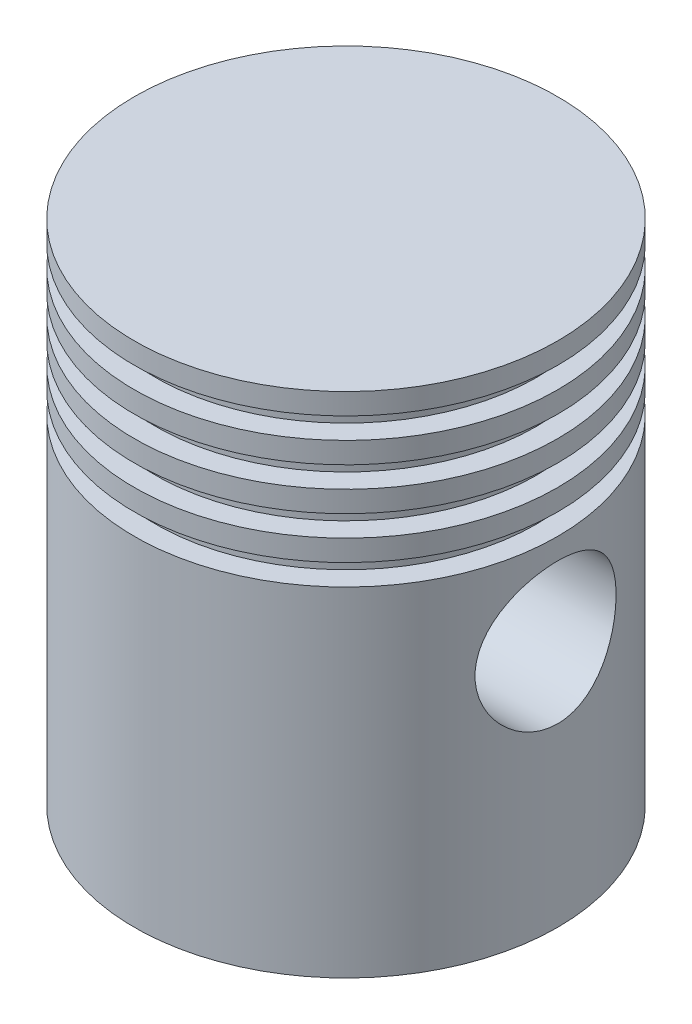
from build123d import *

# Parameters (mm, degrees)
PIN_BORE_SKETCH_R         = 10
GUDGEON_PIN_BORE_20_DEPTH = 66
EDGE_CHAMFER_2X45_SIZE    = 2
INNER_CAVITY_SKETCH_W     = 20
INNER_CAVITY_SKETCH_H     = 29
INNER_CAVITY_CUT_DEPTH    = 48


with BuildPart() as part:
    # Piston Profile Sketch → Piston Body Revolve (revolve)
    with BuildSketch(Plane.XY, mode=Mode.PRIVATE) as piston_body_revolve_sk:
        Polygon((-24, 0), (-30, 0), (-30, 48), (-27, 48), (-27, 51), (-30, 51), (-30, 54), (-27, 54), (-27, 57), (-30, 57), (-30, 60), (-27, 60), (-27, 63), (-30, 63), (-30, 66), (-27, 66), (-27, 69), (-30, 69), (-30, 72), (0, 72), (0, 60), (-24, 60), (-24, 48), (-10, 48), (-10, 22), (-24, 22), align=None)
    revolve(piston_body_revolve_sk.sketch.rotate(Axis((0, 60, 0), (0, 1, 0)), 180), axis=Axis((0, 60, 0), (0, 1, 0)))

    # Pin Bore Sketch → Gudgeon Pin Bore Ø20 (cut, symmetric)
    with BuildSketch(Plane(origin=(0, 0, 0), x_dir=(0, 0, -1), z_dir=(1, 0, 0))):
        with Locations(Location((0, 35, 0), (0, 0, 270))):
            Circle(PIN_BORE_SKETCH_R)
    extrude(amount=GUDGEON_PIN_BORE_20_DEPTH, both=True, mode=Mode.SUBTRACT)

    # Edge Chamfer 2x45°
    edge_chamfer_2x45_edges = [part.edges().sort_by_distance(p)[0] for p in [
        (-24, 0, 0),
    ]]
    chamfer(edge_chamfer_2x45_edges, length=EDGE_CHAMFER_2X45_SIZE)

    # Inner Cavity Sketch → Inner Cavity Cut (cut)
    with BuildSketch(Plane.XZ):
        Rectangle(INNER_CAVITY_SKETCH_W, INNER_CAVITY_SKETCH_H)
    extrude(amount=-INNER_CAVITY_CUT_DEPTH, mode=Mode.SUBTRACT)


solid = part.part
